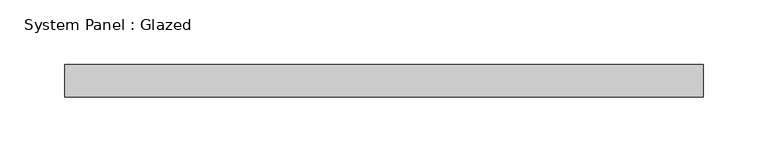
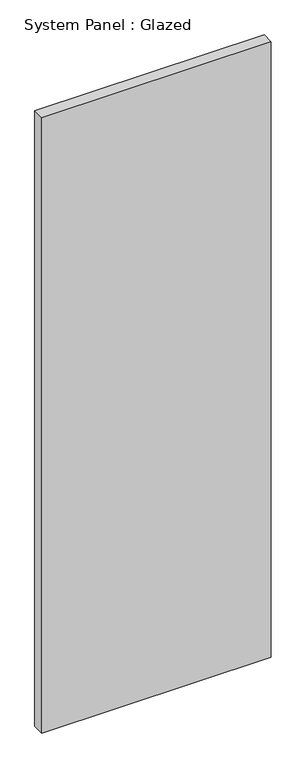
"""IFC4 building model written with IfcOpenShell, lengths in millimetres: plate geometry, System Panel : Glazed."""

from ifc_helpers import new_model, si_unit, origin, origin_with_axes, place, context, project, spatial, polyline, outline, extrude, source, transform, mapped, element, save


def system_panel_glazed_6a435647(model_context):
    return source(origin(), model_context, "Body", "SweptSolid", [
        extrude(outline(polyline([(247.65, 19.05), (-247.65, 19.05), (-247.65, 44.45), (247.65, 44.45), (247.65, 19.05)])), origin_with_axes(), (0.0, 0.0, 1.0), 1402.3594037),
    ])


if __name__ == "__main__":
    model = new_model("IFC4")
    model_context = context("Model", 3, world=origin())
    ifc_project = project(units=[si_unit("LENGTHUNIT", "METRE", prefix="MILLI")], contexts=[model_context])
    site = spatial("IfcSite", under=ifc_project)
    building = spatial("IfcBuilding", under=site)
    placement = place(None, origin())
    system_panel_glazed_shape = system_panel_glazed_6a435647(model_context)
    element("IfcPlate", 1, ObjectType="System Panel : Glazed", at=placement, inside=building, context=model_context, shape_type="MappedRepresentation", body=[
        mapped(system_panel_glazed_shape, transform((0.0, 0.0, 0.0), x_axis=(1.0, 0.0, 0.0), y_axis=(0.0, 1.0, 0.0), z_axis=(0.0, 0.0, 1.0))),
    ])
    save(model, "model.ifc")

# Revit data of these elements
# Type "System Panel : Glazed"
#   Construction Type Id = "GSP4R"
#   Analytic Construction = "1/8 in Pilkington single glazing"
#   Visual Light Transmittance = 0.9
#   Solar Heat Gain Coefficient = 0.86
#   Heat Transfer Coefficient (U) = 1.18115 BTU/(h·ft²·°F)
#   Define Thermal Properties by = 1
# Element 1 (IfcPlate, "System Panel : Glazed")
#   Materials on its faces: "Glass"
# Materials
#   "Glass": class "Glass", colour RGB 0 128 192, transparency 0.75, Description = "Soda Lime Glass", Cost = 0
